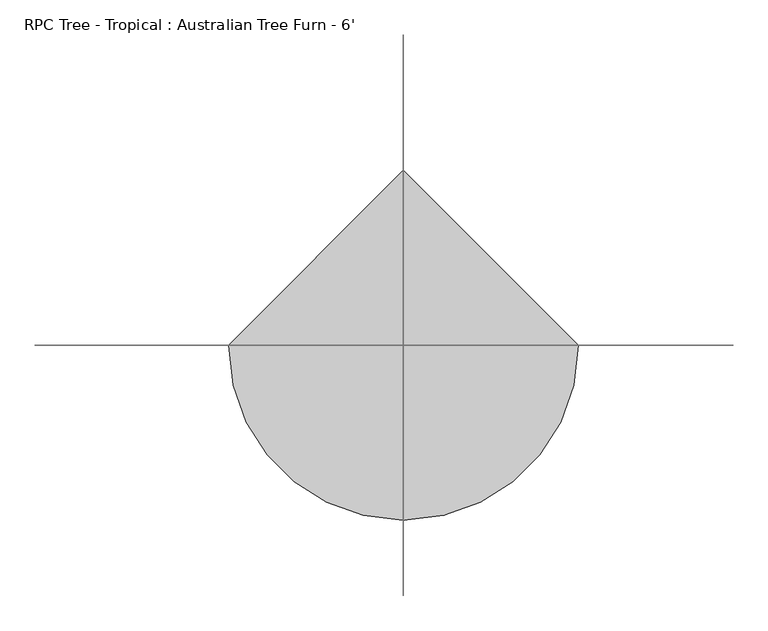
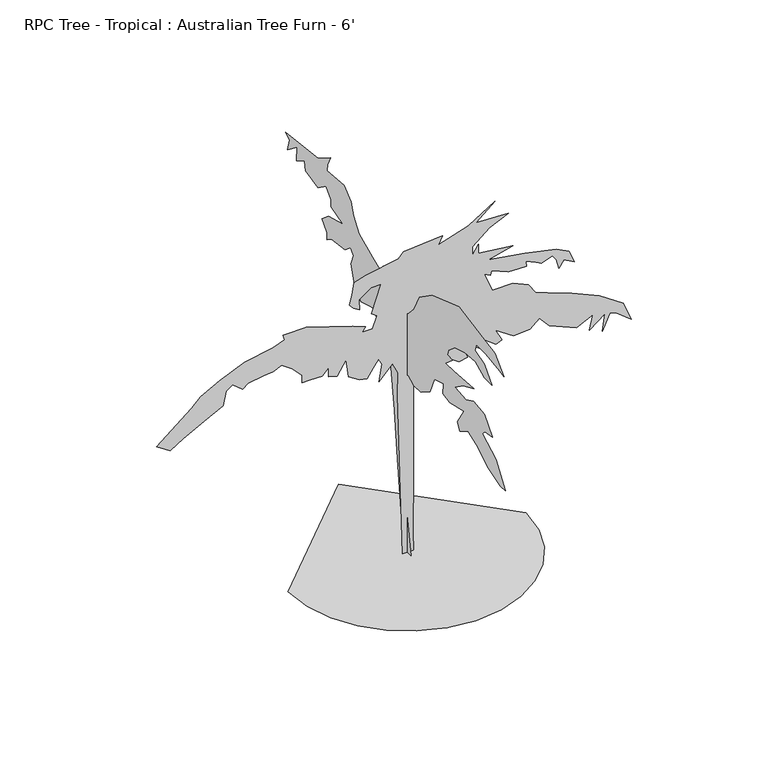
"""IFC4 building model written with IfcOpenShell, lengths in millimetres: geographic element geometry, RPC Tree - Tropical : Australian Tree Furn - 6'."""

from ifc_helpers import new_model, si_unit, origin, place, context, project, spatial, triangles, source, transform, mapped, element, save


def rpc_tree_tropical_australian_tree_furn_6_77f1a640(model_context):
    return source(origin(), model_context, "Body", "Tessellation", [
        triangles([(-639.0365753, 0.0, 0.0007159), (-622.1405136, -146.4247652, 0.0007159), (-574.0277527, -280.8912123, 0.0007159), (-498.5465315, -399.5499215, 0.0007159), (-399.5499215, -498.5465315, 0.0007159), (-280.8912123, -574.0277527, 0.0007159), (-146.4247652, -622.1405136, 0.0007159), (2.79e-05, -639.0365753, 0.0007159), (146.4247652, -622.1429844, 0.0007159), (280.8912123, -574.0277527, 0.0007159), (399.5499215, -498.5465315, 0.0007159), (498.5465315, -399.5499215, 0.0007159), (574.0277527, -280.8912123, 0.0007159), (622.1405136, -146.4247652, 0.0007159), (639.0365753, 5.59e-05, 0.0007159), (-8.38e-05, 639.0365753, 0.0007159), (470.2991641, -3.5e-05, 1828.8014534), (368.5593713, -2.98e-05, 1741.5955845), (542.9711454, -2.94e-05, 1734.3285862), (441.231389, -2.66e-05, 1687.0922253), (350.3907492, -2.2e-05, 1610.7880165), (350.3907492, -1.92e-05, 1563.5516556), (383.0932589, -2.22e-05, 1614.4202076), (383.0932589, -1.92e-05, 1563.5516556), (568.4067295, -1.79e-05, 1541.750806), (437.5966181, -1.59e-05, 1509.0482964), (633.8092781, -1.4e-05, 1476.3456413), (800.9540903, -1.18e-05, 1440.0109406), (869.9913008, -9.7e-06, 1403.673769), (899.0591486, -5.5e-06, 1334.6364132), (840.9235256, -7.5e-06, 1367.3389229), (815.4879416, -5.1e-06, 1327.3695602), (800.9540903, -8.4e-06, 1381.8729195), (779.1532408, -1.01e-05, 1410.9406219), (721.015147, -8.8e-06, 1389.1397724), (691.9473719, -9.7e-06, 1403.673769), (637.4440126, -1.12e-05, 1429.1092804), (641.0762037, -9.4e-06, 1400.0414326), (597.4745047, -9.4e-06, 1400.0414326), (542.9711454, -9.7e-06, 1403.673769), (452.1330491, -1.18e-05, 1440.0109406), (448.4983146, -1.03e-05, 1414.5754292), (415.7958049, -1.14e-05, 1432.7440876), (459.4000111, -5.1e-06, 1327.3695602), (568.4067295, -5.1e-06, 1327.3695602), (651.9778639, -2.9e-06, 1291.0347141), (688.3126373, 3e-07, 1236.5313549), (753.7176567, 1.8e-06, 1211.0958435), (884.5252247, 4.9e-06, 1160.2246754), (1033.5014511, 8.7e-06, 1094.8221268), (1160.6767553, 1.39e-05, 1007.6162579), (1204.2784544, 2.02e-05, 902.2417305), (1120.70732, 1.63e-05, 967.6468225), (1088.0048103, 1.59e-05, 974.9137482), (1048.0353024, 2.11e-05, 887.7078793), (1062.5692263, 1.55e-05, 982.1806738), (978.9980919, 1.94e-05, 916.7781979), (997.1666777, 1.44e-05, 1000.3493322), (909.9608088, 1.7e-05, 956.7450897), (764.6193169, 1.33e-05, 1018.5179907), (710.1159576, 9.6e-06, 1080.2882755), (659.2448622, 1.22e-05, 1036.684033), (572.0389206, 1.26e-05, 1029.4171074), (473.9338986, 8.7e-06, 1094.8221268), (510.2686357, 1.26e-05, 1029.4171074), (477.5660897, 1.35e-05, 1014.8831835), (324.9577085, 6.6e-06, 1131.1569002), (419.4305394, 1.44e-05, 1000.3493322), (284.9882369, 8.7e-06, 1094.8221268), (324.9577085, 1.48e-05, 993.0824066), (277.7212749, 1.52e-05, 985.8154083), (190.5151335, 1.16e-05, 1047.5857658), (88.7756132, 9.6e-06, 1080.2882755), (194.1488688, 1.52e-05, 985.8154083), (30.6385209, 1.11e-05, 1054.8526915), (34.2719928, 1.57e-05, 978.5484827), (34.2719928, 3.32e-05, 684.2282936), (34.2719928, 4.84e-05, 429.8801196), (30.6385209, 6.77e-05, 106.4923825), (34.2719928, 7.35e-05, 0.0013276), (-23.8650472, 7.39e-05, 0.0007003), (-52.9336422, 1.98e-05, 909.5111996), (-49.2999159, 1.22e-05, 1036.684033), (-78.3684632, 8.5e-06, 1098.4543905), (-151.0396997, 1.31e-05, 1022.1501818), (-136.5055487, 7.5e-06, 1116.6229763), (-154.6734259, 5.5e-06, 1149.325486), (-183.7417098, 7.9e-06, 1109.3560507), (-216.4437289, 1.07e-05, 1062.1196171), (-256.4132006, 1.03e-05, 1069.3865427), (-314.5512943, 8.1e-06, 1105.7213161), (-329.0852182, 2e-06, 1207.461109), (-376.3216155, 6.6e-06, 1131.1569002), (-423.5580491, 5.7e-06, 1145.6907515), (-423.5580491, 2.7e-06, 1196.5619196), (-456.2580153, 4.9e-06, 1160.2246754), (-518.0283365, 4.9e-06, 1160.2246754), (-565.2647701, 4.9e-06, 1160.2246754), (-565.2647701, 2.3e-06, 1203.8289179), (-619.7706728, -1e-06, 1258.3322044), (-674.2714886, -3.4e-06, 1298.3017124), (-721.5079222, -2.1e-06, 1276.5008629), (-772.3790903, -1.9e-06, 1272.866201), (-855.9502247, -1e-06, 1258.3322044), (-885.0205433, 3e-07, 1236.5313549), (-939.5239025, -2.3e-06, 1280.133054), (-972.2238688, -8e-07, 1254.6975426), (-990.3925272, 3.8e-06, 1178.3933338), (-1092.13232, 6.8e-06, 1127.5247091), (-1204.773773, 1.05e-05, 1065.7543516), (-1273.8110561, 1.31e-05, 1022.1501818), (-1346.4830738, 1.03e-05, 1069.3865427), (-1157.5373394, 1.2e-06, 1221.9975037), (-1110.3009058, -1.9e-06, 1272.866201), (-1008.561113, -5.1e-06, 1327.3695602), (-874.1188105, -8.6e-06, 1385.5075813), (-721.5079222, -1.03e-05, 1414.5754292), (-659.7375647, -1.16e-05, 1436.3762787), (-667.004563, -1.33e-05, 1465.4439812), (-539.8317295, -1.33e-05, 1465.4439812), (-416.2885437, -1.1e-05, 1425.4770893), (-292.7479377, -8.6e-06, 1385.5075813), (-223.7109271, -7.1e-06, 1360.0720699), (-241.8788043, -5.5e-06, 1334.6364132), (-187.3751907, -5.5e-06, 1334.6364132), (-161.9403697, -9.4e-06, 1400.0414326), (-191.0089079, -1.07e-05, 1421.8422821), (-140.1390206, -1.96e-05, 1570.8185085), (-194.6423889, -1.96e-05, 1570.8185085), (-260.0454098, -1.68e-05, 1523.5821476), (-256.4132006, -1.33e-05, 1465.4439812), (-289.1157284, -1.46e-05, 1487.2474468), (-310.9165598, -1.62e-05, 1512.6804874), (-296.3826722, -1.94e-05, 1567.1838467), (-285.4809939, -2.31e-05, 1628.956675), (-220.0774642, -2.44e-05, 1650.7575245), (-45.666444, -2.63e-05, 1683.4600342), (-20.2313959, -2.81e-05, 1712.5277367), (190.5151335, -2.92e-05, 1730.6963951), (168.7137935, -2.66e-05, 1687.0922253), (328.5898996, -2.96e-05, 1737.9633934), (3.03e-05, -861.8582216, 1549.8330162), (2.4e-05, -733.5424347, 1570.5289913), (2.01e-05, -646.6209961, 1570.5289913), (2.06e-05, -630.0627771, 1529.1370411), (2.54e-05, -721.12437, 1504.3009117), (3.07e-05, -787.3523769, 1425.6574562), (2.76e-05, -716.9866865, 1425.6574562), (2.26e-05, -634.2029314, 1467.0492611), (1.86e-05, -539.0011479, 1458.7689526), (1.52e-05, -443.8018716, 1429.7951397), (1.41e-05, -385.8542459, 1380.1253517), (1.46e-05, -373.4361812, 1347.0113846), (1.68e-05, -423.1059328, 1347.0113846), (1.55e-05, -356.8778895, 1289.0637589), (1.89e-05, -435.5239975, 1293.2039131), (2.69e-05, -621.7848667, 1305.6220505), (2.36e-05, -518.3052092, 1260.089946), (2.19e-05, -443.8018716, 1206.2800037), (2.68e-05, -547.2815291, 1198.0020933), (2.89e-05, -617.6471832, 1231.1161331), (3.37e-05, -716.9866865, 1218.6980684), (3.97e-05, -795.6302147, 1135.9143133), (3.69e-05, -725.2645243, 1123.4987921), (3.66e-05, -700.4309383, 1098.6626627), (4.42e-05, -824.6040276, 1028.2969723), (5.2e-05, -915.6656204, 904.1213396), (4.99e-05, -865.9959051, 899.9836561), (4.34e-05, -745.9604994, 937.2353794), (3.69e-05, -642.4808418, 999.3231594), (3.26e-05, -567.9774679, 1032.4371992), (3.06e-05, -489.3313963, 982.7648678), (2.84e-05, -468.6354575, 1024.1567453), (2.82e-05, -530.7232738, 1123.4987921), (2.33e-05, -398.2697671, 1090.3847523), (2e-05, -332.0443036, 1102.802817), (1.84e-05, -336.1819871, 1160.7504427), (1.55e-05, -253.3997399, 1135.9143133), (1.65e-05, -212.0081348, 1040.715037), (1.44e-05, -129.2246341, 986.9050947), (1.15e-05, -62.9981487, 982.7648678), (8.4e-06, -13.3280768, 1011.7412241), (6.8e-06, 32.2026538, 999.3231594), (4.5e-06, 52.8985925, 1044.8527205), (4.9e-06, 81.8726461, 986.9050947), (7e-06, 86.0118375, 912.3991774), (1.57e-05, 57.0377794, 664.0505281), (2.77e-05, 19.7852431, 316.3597959), (3.93e-05, -34.0238362, 0.0007149), (3.64e-05, 36.3418406, 0.0), (3.07e-05, 52.8985925, 167.3503229), (1.97e-05, 90.1512742, 477.7870791), (1.08e-05, 119.1250779, 734.4162186), (1.5e-06, 156.3777732, 991.0453217), (-4.8e-06, 210.1869524, 1119.3585651), (-7.3e-06, 268.135323, 1119.3585651), (-1.14e-05, 305.3869918, 1198.0020933), (-1.38e-05, 371.6149987, 1181.4464178), (-1.58e-05, 429.5625881, 1160.7504427), (-2.04e-05, 491.6504045, 1222.8382954), (-2.47e-05, 520.6242173, 1322.177726), (-2.55e-05, 499.9282785, 1380.1253517), (-2.76e-05, 528.9020914, 1409.0991646), (-2.86e-05, 578.5718067, 1367.7072144), (-3.37e-05, 702.7474394, 1351.1515388), (-3.47e-05, 744.1393169, 1322.177726), (-3.59e-05, 744.1393169, 1363.5696762), (-3.96e-05, 793.8090322, 1413.2393188), (-3.83e-05, 731.7212523, 1462.9091068), (-3.35e-05, 599.2677455, 1500.1607574), (-3.93e-05, 706.8876663, 1533.2747246), (-4.06e-05, 711.0252771, 1570.5289913), (-4.41e-05, 756.5573816, 1620.1987793), (-4.58e-05, 831.0607555, 1566.3888371), (-5.18e-05, 946.9584778, 1591.2223503), (-5.36e-05, 955.2363155, 1640.8946091), (-5.57e-05, 1029.7422329, 1599.5028042), (-5.79e-05, 1025.602006, 1678.1462597), (-5.98e-05, 1112.525988, 1611.9183254), (-6.09e-05, 1095.9676964, 1674.0061054), (-6.33e-05, 1133.2218904, 1698.8422348), (-5.08e-05, 831.0607555, 1731.9562019), (-4.78e-05, 715.1655041, 1806.4596485), (-4.73e-05, 739.99909, 1752.652177), (-4.64e-05, 748.2795439, 1711.2603722), (-3.97e-05, 586.8496808, 1727.8160477), (-3.52e-05, 520.6242173, 1674.0061054), (-3.23e-05, 499.9282785, 1607.7806419), (-2.78e-05, 446.1183363, 1537.4150242), (-2.05e-05, 321.9452471, 1479.4647823), (-1.04e-05, 143.960199, 1409.0991646), (-1.65e-05, 226.7434454, 1487.7452362), (-9.7e-06, 114.9858956, 1429.7951397), (-2.2e-06, -0.9105653, 1351.1515388), (-1.4e-06, -62.9981487, 1417.3796185), (-2.2e-06, -112.668141, 1516.7190491), (7e-07, -232.7038011, 1599.5028042), (9.2e-06, -481.0535222, 1686.4242428), (2.03e-05, -700.4309383, 1645.0322926), (2.61e-05, -816.3261898, 1624.3363174), (3.23e-05, -899.1099449, 1541.5525623)], [[15, 16, 1], [14, 15, 1], [14, 1, 2], [13, 14, 2], [13, 2, 3], [13, 3, 4], [12, 13, 4], [11, 12, 4], [11, 4, 5], [11, 5, 6], [11, 6, 7], [11, 7, 8], [11, 8, 9], [11, 9, 10], [141, 17, 18], [54, 55, 56], [73, 74, 75], [67, 68, 69], [24, 25, 26], [18, 19, 20], [51, 52, 53], [22, 23, 24], [84, 85, 86], [29, 30, 31], [56, 57, 58], [31, 32, 33], [130, 131, 132], [138, 139, 140], [41, 42, 43], [111, 112, 113], [110, 111, 113], [109, 110, 113], [122, 123, 124], [118, 119, 120], [18, 20, 21], [141, 18, 21], [69, 70, 71], [69, 71, 72], [28, 29, 31], [28, 31, 33], [28, 33, 34], [27, 28, 34], [27, 34, 35], [27, 35, 36], [27, 36, 37], [130, 132, 133], [130, 133, 134], [50, 51, 53], [50, 53, 54], [50, 54, 56], [50, 56, 58], [140, 141, 21], [37, 38, 39], [64, 65, 66], [64, 66, 67], [80, 81, 82], [79, 80, 82], [78, 79, 82], [77, 78, 82], [76, 77, 82], [76, 82, 83], [75, 76, 83], [97, 98, 99], [49, 50, 58], [49, 58, 59], [49, 59, 60], [48, 49, 60], [48, 60, 61], [47, 48, 61], [129, 130, 134], [129, 134, 135], [129, 135, 136], [129, 136, 137], [128, 129, 137], [108, 109, 113], [108, 113, 114], [107, 108, 114], [107, 114, 115], [106, 107, 115], [106, 115, 116], [105, 106, 116], [104, 105, 116], [103, 104, 116], [103, 116, 117], [102, 103, 117], [101, 102, 117], [101, 117, 118], [75, 83, 84], [26, 27, 37], [26, 37, 39], [26, 39, 40], [26, 40, 41], [26, 41, 43], [92, 93, 94], [92, 94, 95], [126, 127, 128], [101, 118, 120], [100, 101, 120], [100, 120, 121], [99, 100, 121], [97, 99, 121], [96, 97, 121], [95, 96, 121], [95, 121, 122], [92, 95, 122], [92, 122, 124], [140, 21, 22], [88, 89, 90], [24, 26, 43], [22, 24, 43], [88, 90, 91], [88, 91, 92], [88, 92, 124], [87, 88, 124], [87, 124, 125], [47, 61, 62], [47, 62, 63], [47, 63, 64], [46, 47, 64], [45, 46, 64], [44, 45, 64], [44, 64, 67], [43, 44, 67], [137, 138, 140], [128, 137, 140], [126, 128, 140], [126, 140, 22], [126, 22, 43], [126, 43, 67], [126, 67, 69], [126, 69, 72], [126, 72, 73], [125, 126, 73], [87, 125, 73], [87, 73, 75], [87, 75, 84], [87, 84, 86], [231, 232, 233], [156, 157, 158], [240, 241, 142], [222, 223, 224], [218, 219, 220], [220, 221, 222], [218, 220, 222], [153, 154, 155], [240, 142, 143], [239, 240, 143], [146, 147, 148], [205, 206, 207], [162, 163, 164], [156, 158, 159], [216, 217, 218], [216, 218, 222], [166, 167, 168], [166, 168, 169], [222, 224, 225], [239, 143, 144], [238, 239, 144], [146, 148, 149], [145, 146, 149], [165, 166, 169], [165, 169, 170], [207, 208, 209], [188, 189, 190], [188, 190, 191], [188, 191, 192], [187, 188, 192], [187, 192, 193], [186, 187, 193], [186, 193, 194], [185, 186, 194], [171, 172, 173], [171, 173, 174], [145, 149, 150], [155, 156, 159], [165, 170, 171], [165, 171, 174], [175, 176, 177], [182, 183, 184], [205, 207, 209], [205, 209, 210], [204, 205, 210], [203, 204, 210], [161, 162, 164], [161, 164, 165], [161, 165, 174], [160, 161, 174], [159, 160, 174], [159, 174, 175], [159, 175, 177], [155, 159, 177], [238, 144, 145], [238, 145, 150], [237, 238, 150], [237, 150, 151], [237, 151, 152], [236, 237, 152], [235, 236, 152], [235, 152, 153], [235, 153, 155], [235, 155, 177], [235, 177, 178], [234, 235, 178], [234, 178, 179], [234, 179, 180], [234, 180, 181], [234, 181, 182], [234, 182, 184], [231, 233, 234], [231, 234, 184], [214, 215, 216], [214, 216, 222], [213, 214, 222], [213, 222, 225], [213, 225, 226], [212, 213, 226], [212, 226, 227], [212, 227, 228], [211, 212, 228], [210, 211, 228], [210, 228, 229], [203, 210, 229], [203, 229, 230], [202, 203, 230], [184, 185, 194], [184, 194, 195], [231, 184, 195], [230, 231, 195], [230, 195, 196], [230, 196, 197], [202, 230, 197], [202, 197, 198], [201, 202, 198], [200, 201, 198], [199, 200, 198]], closed=False),
    ])


if __name__ == "__main__":
    model = new_model("IFC4")
    model_context = context("Model", 3, world=origin())
    ifc_project = project(units=[si_unit("LENGTHUNIT", "METRE", prefix="MILLI")], contexts=[model_context])
    site = spatial("IfcSite", under=ifc_project)
    building = spatial("IfcBuilding", under=site)
    placement = place(None, origin())
    rpc_tree_tropical_australian_tree_furn_6_shape = rpc_tree_tropical_australian_tree_furn_6_77f1a640(model_context)
    element("IfcGeographicElement", 1, ObjectType="RPC Tree - Tropical : Australian Tree Furn - 6'", at=placement, inside=building, context=model_context, shape_type="MappedRepresentation", body=[
        mapped(rpc_tree_tropical_australian_tree_furn_6_shape, transform((0.0, 0.0, 0.0), x_axis=(1.0, 0.0, 0.0), y_axis=(0.0, 1.0, 0.0), z_axis=(0.0, 0.0, 1.0))),
    ])
    save(model, "model.ifc")

# Revit data of these elements
# Type "RPC Tree - Tropical : Australian Tree Furn - 6'"
#   built-in parameter 1005198 = "{2, 15},{39, RPC-16-FVCN-UWG0-AP53-A000-ST1L-LVER-AU},{1, 0},{1, 0},{2, 13},{1, 8},{5, Color},{1, 0},{1, 0},{3, 0.8},{3, 0.8},{3, 0.8},{1, 8},{7, BBoxMin},{1, 0},{1, 0},{1, 0},{1, 0},{1, 0},{1, 8},{7, BBoxMax},{1, 0},{1, 0},{1, 0},{1, 0},{1, 0},{2, 11},{9, RPCTypeId},{1, 0},{1, 0},{39, RPC-16-FVCN-UWG0-AP53-A000-ST1L-LVER-AU},{1, 6},{14, RPCPlantHeight},{1, 0},{1, 0},{1, 6},{2, 11},{7, keyword},{1, 0},{1, 0},{35, :RPCs:Trees [Tropical]:Geometry:RPC},{2, 11},{8, category},{1, 0},{1, 0},{16, Trees [Tropical]},{2, 11},{12, LocalizedUID},{1, 0},{1, 0},{20, Australian Tree Fern},{2, 14},{6, Height},{1, 0},{1, 0},{1, 6},{1, 2},{16, Cast Reflections},{1, 0},{1, 0},{1, 0},{1, 2},{12, Cast Shadows},{1, 0},{1, 0},{1, 1},{1, 2},{9, Lock View},{1, 0},{1, 0},{1, 0},{1, 4},{5, ViewC},{1, 0},{1, 0},{1, 0},{21, assetlibrary_base.fbx},{1, 5},"
#   built-in parameter 1005195 = "RPC-16-FVCN-UWG0-AP53-A000-ST1L-LVER-AU"
#   Type Comments = "Australian Tree Furn"
#   Assembly Code = "G2050500"
#   Height = 6' - 0"
#   Plan Symbol = element 354646
#   Default Elevation = 0
